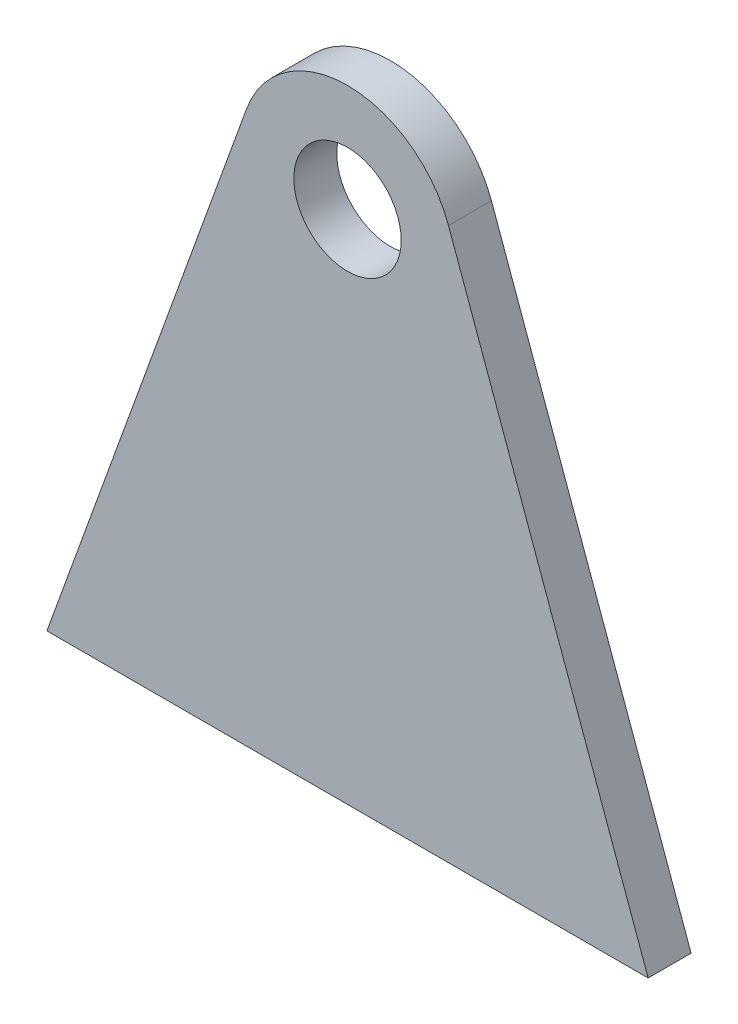
ISO-10303-21;
HEADER;
FILE_DESCRIPTION(('STEP AP214'),'2;1');
FILE_NAME('part.step','',(''),(''),'','','');
FILE_SCHEMA(('AUTOMOTIVE_DESIGN { 1 0 10303 214 1 1 1 1 }'));
ENDSEC;
DATA;
#1=APPLICATION_CONTEXT('core data for automotive mechanical design processes');
#2=APPLICATION_PROTOCOL_DEFINITION('international standard','automotive_design',2000,#1);
#3=PRODUCT_CONTEXT('',#1,'mechanical');
#4=PRODUCT('Part','Part','',(#3));
#5=PRODUCT_RELATED_PRODUCT_CATEGORY('part','',(#4));
#6=PRODUCT_DEFINITION_FORMATION('','',#4);
#7=PRODUCT_DEFINITION_CONTEXT('part definition',#1,'design');
#8=PRODUCT_DEFINITION('design','',#6,#7);
#9=PRODUCT_DEFINITION_SHAPE('','',#8);
#10=(LENGTH_UNIT() NAMED_UNIT(*) SI_UNIT(.MILLI.,.METRE.));
#11=(NAMED_UNIT(*) PLANE_ANGLE_UNIT() SI_UNIT($,.RADIAN.));
#12=(NAMED_UNIT(*) SI_UNIT($,.STERADIAN.) SOLID_ANGLE_UNIT());
#13=UNCERTAINTY_MEASURE_WITH_UNIT(LENGTH_MEASURE(1.E-05),#10,'distance_accuracy_value','');
#14=(GEOMETRIC_REPRESENTATION_CONTEXT(3) GLOBAL_UNCERTAINTY_ASSIGNED_CONTEXT((#13)) GLOBAL_UNIT_ASSIGNED_CONTEXT((#10,
#11,#12)) REPRESENTATION_CONTEXT('',''));
#15=CARTESIAN_POINT('',(0.,0.,0.));
#16=DIRECTION('',(0.,0.,1.));
#17=DIRECTION('',(1.,0.,0.));
#18=AXIS2_PLACEMENT_3D('',#15,#16,#17);
#19=CARTESIAN_POINT('',(0.,0.,20.));
#20=DIRECTION('',(0.,0.,1.));
#21=DIRECTION('',(1.,0.,0.));
#22=AXIS2_PLACEMENT_3D('',#19,#20,#21);
#23=PLANE('',#22);
#24=DIRECTION('',(-0.340204935652928,-0.940351318262163,0.));
#25=VECTOR('',#24,1.);
#26=CARTESIAN_POINT('',(-47.0175659131081,17.0102467826464,20.));
#27=LINE('',#26,#25);
#28=CARTESIAN_POINT('',(-47.0175659131081,17.0102467826464,20.));
#29=VERTEX_POINT('',#28);
#30=CARTESIAN_POINT('',(-140.,-240.,20.));
#31=VERTEX_POINT('',#30);
#32=EDGE_CURVE('E93',#29,#31,#27,.T.);
#33=ORIENTED_EDGE('',*,*,#32,.T.);
#34=DIRECTION('',(1.,0.,0.));
#35=VECTOR('',#34,1.);
#36=CARTESIAN_POINT('',(-140.,-240.,20.));
#37=LINE('',#36,#35);
#38=CARTESIAN_POINT('',(140.,-240.,20.));
#39=VERTEX_POINT('',#38);
#40=EDGE_CURVE('E88',#31,#39,#37,.T.);
#41=ORIENTED_EDGE('',*,*,#40,.T.);
#42=DIRECTION('',(-0.340204935652928,0.940351318262163,0.));
#43=VECTOR('',#42,1.);
#44=CARTESIAN_POINT('',(47.0175659131081,17.0102467826464,20.));
#45=LINE('',#44,#43);
#46=CARTESIAN_POINT('',(47.0175659131081,17.0102467826464,20.));
#47=VERTEX_POINT('',#46);
#48=EDGE_CURVE('E90',#39,#47,#45,.T.);
#49=ORIENTED_EDGE('',*,*,#48,.T.);
#50=CARTESIAN_POINT('',(0.,0.,20.));
#51=DIRECTION('',(0.,0.,1.));
#52=DIRECTION('',(1.,0.,0.));
#53=AXIS2_PLACEMENT_3D('',#50,#51,#52);
#54=CIRCLE('',#53,50.);
#55=EDGE_CURVE('E57',#47,#29,#54,.T.);
#56=ORIENTED_EDGE('',*,*,#55,.T.);
#57=EDGE_LOOP('',(#33,#41,#49,#56));
#58=FACE_BOUND('',#57,.T.);
#59=CARTESIAN_POINT('',(0.,0.,20.));
#60=DIRECTION('',(0.,0.,1.));
#61=DIRECTION('',(1.,0.,0.));
#62=AXIS2_PLACEMENT_3D('',#59,#60,#61);
#63=CIRCLE('',#62,25.);
#64=CARTESIAN_POINT('',(25.,0.,20.));
#65=VERTEX_POINT('',#64);
#66=EDGE_CURVE('E106',#65,#65,#63,.T.);
#67=ORIENTED_EDGE('',*,*,#66,.F.);
#68=EDGE_LOOP('',(#67));
#69=FACE_BOUND('',#68,.T.);
#70=ADVANCED_FACE('F39',(#58,#69),#23,.T.);
#71=CARTESIAN_POINT('',(0.,0.,0.));
#72=DIRECTION('',(0.,0.,1.));
#73=DIRECTION('',(1.,0.,0.));
#74=AXIS2_PLACEMENT_3D('',#71,#72,#73);
#75=PLANE('',#74);
#76=DIRECTION('',(-0.340204935652928,-0.940351318262163,0.));
#77=VECTOR('',#76,1.);
#78=CARTESIAN_POINT('',(-47.0175659131081,17.0102467826464,0.));
#79=LINE('',#78,#77);
#80=CARTESIAN_POINT('',(-47.0175659131081,17.0102467826464,0.));
#81=VERTEX_POINT('',#80);
#82=CARTESIAN_POINT('',(-140.,-240.,0.));
#83=VERTEX_POINT('',#82);
#84=EDGE_CURVE('E103',#81,#83,#79,.T.);
#85=ORIENTED_EDGE('',*,*,#84,.F.);
#86=CARTESIAN_POINT('',(0.,0.,0.));
#87=DIRECTION('',(0.,0.,1.));
#88=DIRECTION('',(1.,0.,0.));
#89=AXIS2_PLACEMENT_3D('',#86,#87,#88);
#90=CIRCLE('',#89,50.);
#91=CARTESIAN_POINT('',(47.0175659131081,17.0102467826464,0.));
#92=VERTEX_POINT('',#91);
#93=EDGE_CURVE('E78',#92,#81,#90,.T.);
#94=ORIENTED_EDGE('',*,*,#93,.F.);
#95=DIRECTION('',(-0.340204935652928,0.940351318262163,0.));
#96=VECTOR('',#95,1.);
#97=CARTESIAN_POINT('',(47.0175659131081,17.0102467826464,0.));
#98=LINE('',#97,#96);
#99=CARTESIAN_POINT('',(140.,-240.,0.));
#100=VERTEX_POINT('',#99);
#101=EDGE_CURVE('E71',#100,#92,#98,.T.);
#102=ORIENTED_EDGE('',*,*,#101,.F.);
#103=DIRECTION('',(1.,0.,0.));
#104=VECTOR('',#103,1.);
#105=CARTESIAN_POINT('',(-140.,-240.,0.));
#106=LINE('',#105,#104);
#107=EDGE_CURVE('E92',#83,#100,#106,.T.);
#108=ORIENTED_EDGE('',*,*,#107,.F.);
#109=EDGE_LOOP('',(#85,#94,#102,#108));
#110=FACE_BOUND('',#109,.T.);
#111=CARTESIAN_POINT('',(0.,0.,0.));
#112=DIRECTION('',(0.,0.,1.));
#113=DIRECTION('',(1.,0.,0.));
#114=AXIS2_PLACEMENT_3D('',#111,#112,#113);
#115=CIRCLE('',#114,25.);
#116=CARTESIAN_POINT('',(25.,0.,0.));
#117=VERTEX_POINT('',#116);
#118=EDGE_CURVE('E120',#117,#117,#115,.T.);
#119=ORIENTED_EDGE('',*,*,#118,.T.);
#120=EDGE_LOOP('',(#119));
#121=FACE_BOUND('',#120,.T.);
#122=ADVANCED_FACE('F111',(#110,#121),#75,.F.);
#123=CARTESIAN_POINT('',(-47.0175659131081,17.0102467826464,20.));
#124=DIRECTION('',(0.940351318262163,-0.340204935652928,0.));
#125=DIRECTION('',(0.340204935652928,0.940351318262163,0.));
#126=AXIS2_PLACEMENT_3D('',#123,#124,#125);
#127=PLANE('',#126);
#128=ORIENTED_EDGE('',*,*,#84,.T.);
#129=DIRECTION('',(0.,0.,-1.));
#130=VECTOR('',#129,1.);
#131=CARTESIAN_POINT('',(-140.,-240.,20.));
#132=LINE('',#131,#130);
#133=EDGE_CURVE('E11',#31,#83,#132,.T.);
#134=ORIENTED_EDGE('',*,*,#133,.F.);
#135=ORIENTED_EDGE('',*,*,#32,.F.);
#136=DIRECTION('',(0.,0.,-1.));
#137=VECTOR('',#136,1.);
#138=CARTESIAN_POINT('',(-47.0175659131081,17.0102467826464,20.));
#139=LINE('',#138,#137);
#140=EDGE_CURVE('E97',#29,#81,#139,.T.);
#141=ORIENTED_EDGE('',*,*,#140,.T.);
#142=EDGE_LOOP('',(#128,#134,#135,#141));
#143=FACE_BOUND('',#142,.T.);
#144=ADVANCED_FACE('F41',(#143),#127,.F.);
#145=CARTESIAN_POINT('',(-140.,-240.,20.));
#146=DIRECTION('',(0.,1.,0.));
#147=DIRECTION('',(0.,0.,1.));
#148=AXIS2_PLACEMENT_3D('',#145,#146,#147);
#149=PLANE('',#148);
#150=ORIENTED_EDGE('',*,*,#107,.T.);
#151=DIRECTION('',(0.,0.,-1.));
#152=VECTOR('',#151,1.);
#153=CARTESIAN_POINT('',(140.,-240.,20.));
#154=LINE('',#153,#152);
#155=EDGE_CURVE('E48',#39,#100,#154,.T.);
#156=ORIENTED_EDGE('',*,*,#155,.F.);
#157=ORIENTED_EDGE('',*,*,#40,.F.);
#158=ORIENTED_EDGE('',*,*,#133,.T.);
#159=EDGE_LOOP('',(#150,#156,#157,#158));
#160=FACE_BOUND('',#159,.T.);
#161=ADVANCED_FACE('F94',(#160),#149,.F.);
#162=CARTESIAN_POINT('',(47.0175659131081,17.0102467826464,20.));
#163=DIRECTION('',(-0.940351318262163,-0.340204935652928,0.));
#164=DIRECTION('',(0.340204935652928,-0.940351318262163,0.));
#165=AXIS2_PLACEMENT_3D('',#162,#163,#164);
#166=PLANE('',#165);
#167=ORIENTED_EDGE('',*,*,#101,.T.);
#168=DIRECTION('',(0.,0.,-1.));
#169=VECTOR('',#168,1.);
#170=CARTESIAN_POINT('',(47.0175659131081,17.0102467826464,20.));
#171=LINE('',#170,#169);
#172=EDGE_CURVE('E96',#47,#92,#171,.T.);
#173=ORIENTED_EDGE('',*,*,#172,.F.);
#174=ORIENTED_EDGE('',*,*,#48,.F.);
#175=ORIENTED_EDGE('',*,*,#155,.T.);
#176=EDGE_LOOP('',(#167,#173,#174,#175));
#177=FACE_BOUND('',#176,.T.);
#178=ADVANCED_FACE('F100',(#177),#166,.F.);
#179=CARTESIAN_POINT('',(0.,0.,20.));
#180=DIRECTION('',(0.,0.,-1.));
#181=DIRECTION('',(-1.,0.,0.));
#182=AXIS2_PLACEMENT_3D('',#179,#180,#181);
#183=CYLINDRICAL_SURFACE('',#182,50.);
#184=ORIENTED_EDGE('',*,*,#93,.T.);
#185=ORIENTED_EDGE('',*,*,#140,.F.);
#186=ORIENTED_EDGE('',*,*,#55,.F.);
#187=ORIENTED_EDGE('',*,*,#172,.T.);
#188=EDGE_LOOP('',(#184,#185,#186,#187));
#189=FACE_BOUND('',#188,.T.);
#190=ADVANCED_FACE('F112',(#189),#183,.T.);
#191=CARTESIAN_POINT('',(0.,0.,20.));
#192=DIRECTION('',(0.,0.,-1.));
#193=DIRECTION('',(-1.,0.,0.));
#194=AXIS2_PLACEMENT_3D('',#191,#192,#193);
#195=CYLINDRICAL_SURFACE('',#194,25.);
#196=ORIENTED_EDGE('',*,*,#66,.T.);
#197=EDGE_LOOP('',(#196));
#198=FACE_BOUND('',#197,.T.);
#199=ORIENTED_EDGE('',*,*,#118,.F.);
#200=EDGE_LOOP('',(#199));
#201=FACE_BOUND('',#200,.T.);
#202=ADVANCED_FACE('F123',(#198,#201),#195,.F.);
#203=CLOSED_SHELL('',(#70,#122,#144,#161,#178,#190,#202));
#204=MANIFOLD_SOLID_BREP('B2',#203);
#205=ADVANCED_BREP_SHAPE_REPRESENTATION('',(#18,#204),#14);
#206=SHAPE_DEFINITION_REPRESENTATION(#9,#205);
ENDSEC;
END-ISO-10303-21;
